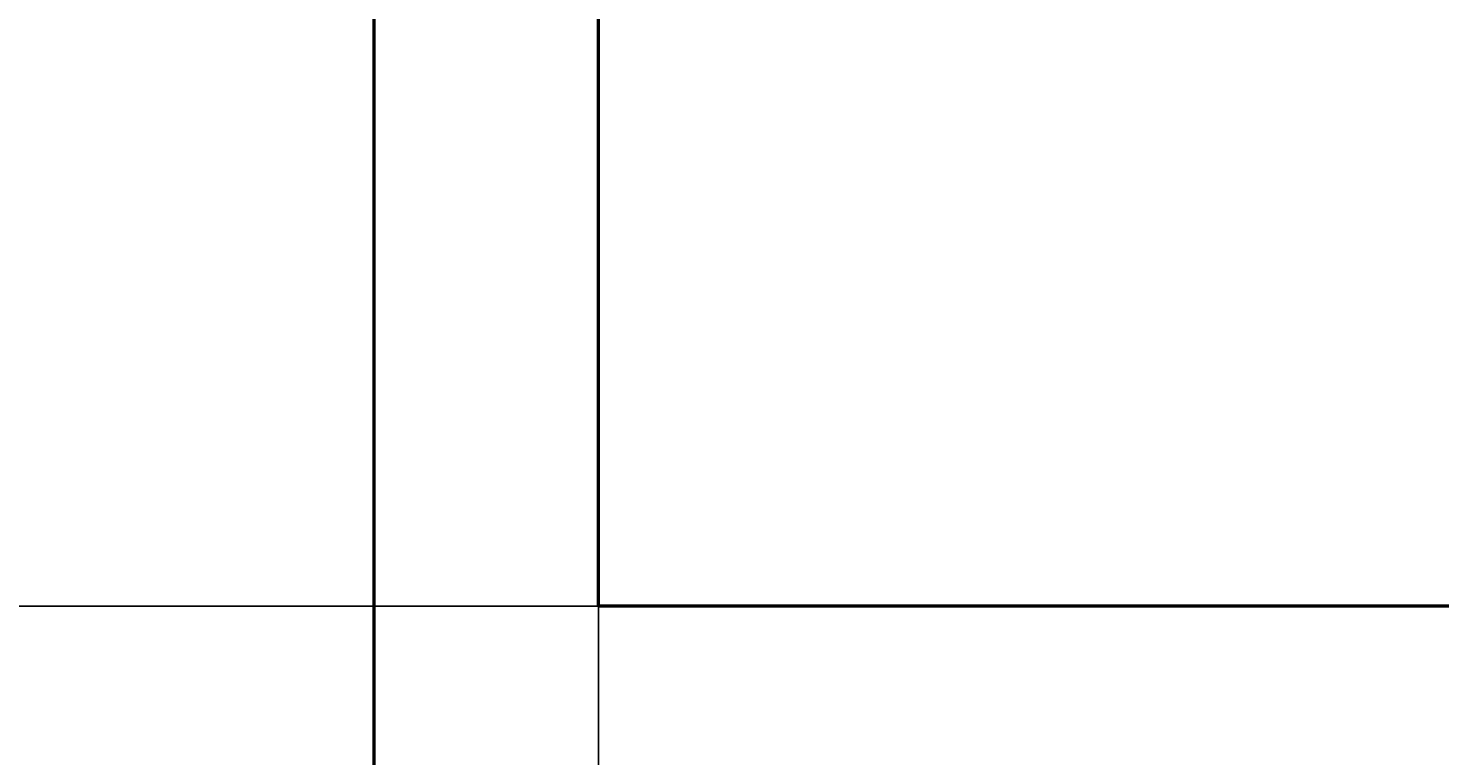
# Model space of a CAD drawing. Units: inches. Extents: x 37 to 824, y -700 to 234.
# Tile 50 of 77: x 147 to 204, y 78 to 107. Entities that reach past the tile are written whole.
import ezdxf

# ---------------------------------------------------------------- set-up
doc = ezdxf.new("R2010")
doc.units = ezdxf.units.IN
doc.header["$MEASUREMENT"] = 0
doc.layers.add('A-ANNO-DIMS', color=2, linetype='Continuous', lineweight=18)
doc.layers.add('A-WALL', color=2, linetype='Continuous', lineweight=50)
doc.styles.get("Standard").update_dxf_attribs({"font": 'arial.ttf'})
doc.dimstyles.get("Standard").update_dxf_attribs({"dimtxt": 0.18, "dimasz": 0.18, "dimexe": 0.18, "dimexo": 0.0625, "dimgap": 0.09, "dimtad": 0, "dimtih": 1, "dimtoh": 1, "dimdec": 1, "dimzin": 0, "dimdsep": 46, "dimlunit": 4, "dimtxsty": 'Standard', "dimcen": 0.09, "dimadec": 0, "dimazin": 0, "dimtfac": 1, "dimtdec": 1, "dimtofl": 0, "dimtmove": 0, "dimatfit": 3, "dimfxl": 1, "dimtolj": 1, "dimtzin": 0, "dimarcsym": 0})

# ---------------------------------------------------------------- blocks, each defined once
blk = doc.blocks.new('*D51')
at = {"layer": 'A-ANNO-DIMS', "color": 0, "lineweight": -2, "ltscale": 0.5, "transparency": 16777216}
for p, q in [((161.015, 113.09), (78.159, 113.09)), ((78.339, 112.91), (78.339, 81.772)), ((78.339, 50.27), (78.339, 81.408)), ((161.015, 50.09), (78.159, 50.09))]:
    blk.add_line(p, q, dxfattribs=at)
at = {"layer": 'A-ANNO-DIMS', "color": 0, "ltscale": 0.5, "transparency": 16777216}
for points in [[(78.309, 112.91), (78.369, 112.91), (78.339, 113.09)], [(78.309, 50.27), (78.369, 50.27), (78.339, 50.09)]]:
    blk.add_solid(points, dxfattribs=at)
at = {"layer": 'Defpoints', "color": 0, "ltscale": 0.5, "transparency": 16777216}
for p in [(161.077, 113.09), (78.339, 50.09), (161.077, 50.09)]:
    blk.add_point(p, dxfattribs=at)
at = {"layer": 'A-ANNO-DIMS', "color": 0, "ltscale": 0.5, "transparency": 16777216, "insert": (78.339, 81.59), "char_height": 0.18, "attachment_point": 5}
blk.add_mtext('\\A1;5\'-3"', dxfattribs=at)
blk = doc.blocks.new('*D60')
at = {"layer": 'A-ANNO-DIMS', "color": 0, "lineweight": -2, "ltscale": 0.5, "transparency": 16777216}
for p, q in [((419.015, 113.09), (78.159, 113.09)), ((78.339, 112.91), (78.339, 98.772)), ((78.339, 84.27), (78.339, 98.409)), ((419.015, 84.09), (78.159, 84.09))]:
    blk.add_line(p, q, dxfattribs=at)
at = {"layer": 'A-ANNO-DIMS', "color": 0, "ltscale": 0.5, "transparency": 16777216}
for points in [[(78.309, 112.91), (78.369, 112.91), (78.339, 113.09)], [(78.309, 84.27), (78.369, 84.27), (78.339, 84.09)]]:
    blk.add_solid(points, dxfattribs=at)
at = {"layer": 'Defpoints', "color": 0, "ltscale": 0.5, "transparency": 16777216}
for p in [(78.339, 113.09), (419.077, 113.09), (419.077, 84.09)]:
    blk.add_point(p, dxfattribs=at)
at = {"layer": 'A-ANNO-DIMS', "color": 0, "ltscale": 0.5, "transparency": 16777216, "insert": (78.339, 98.59), "char_height": 0.18, "attachment_point": 5}
blk.add_mtext('\\A1;2\'-5"', dxfattribs=at)
blk = doc.blocks.new('*D72')
at = {"layer": 'A-ANNO-DIMS', "color": 0, "lineweight": -2, "ltscale": 0.5, "transparency": 16777216}
for p, q in [((170.077, 84.153), (170.077, 234.17)), ((170.257, 233.99), (209.804, 233.99)), ((250.01, 233.99), (210.463, 233.99)), ((250.19, 84.153), (250.19, 234.17))]:
    blk.add_line(p, q, dxfattribs=at)
at = {"layer": 'A-ANNO-DIMS', "color": 0, "ltscale": 0.5, "transparency": 16777216}
for points in [[(170.257, 234.02), (170.257, 233.96), (170.077, 233.99)], [(250.01, 234.02), (250.01, 233.96), (250.19, 233.99)]]:
    blk.add_solid(points, dxfattribs=at)
at = {"layer": 'Defpoints', "color": 0, "ltscale": 0.5, "transparency": 16777216}
for p in [(250.19, 233.99), (170.077, 84.09), (250.19, 84.09)]:
    blk.add_point(p, dxfattribs=at)
at = {"layer": 'A-ANNO-DIMS', "color": 0, "ltscale": 0.5, "transparency": 16777216, "insert": (210.133, 233.99), "char_height": 0.18, "attachment_point": 5}
blk.add_mtext('\\A1;6\'-8"', dxfattribs=at)
blk = doc.blocks.new('*D84')
at = {"layer": 'A-ANNO-DIMS', "color": 0, "lineweight": -2, "ltscale": 0.5, "transparency": 16777216}
for p, q in [((170.077, -265.847), (170.077, 234.17)), ((170.257, 233.99), (189.748, 233.99)), ((209.897, 233.99), (190.406, 233.99)), ((210.077, -265.847), (210.077, 234.17))]:
    blk.add_line(p, q, dxfattribs=at)
at = {"layer": 'A-ANNO-DIMS', "color": 0, "ltscale": 0.5, "transparency": 16777216}
for points in [[(170.257, 234.02), (170.257, 233.96), (170.077, 233.99)], [(209.897, 234.02), (209.897, 233.96), (210.077, 233.99)]]:
    blk.add_solid(points, dxfattribs=at)
at = {"layer": 'Defpoints', "color": 0, "ltscale": 0.5, "transparency": 16777216}
for p in [(210.077, 233.99), (170.077, -265.91), (210.077, -265.91)]:
    blk.add_point(p, dxfattribs=at)
at = {"layer": 'A-ANNO-DIMS', "color": 0, "ltscale": 0.5, "transparency": 16777216, "insert": (190.077, 233.99), "char_height": 0.18, "attachment_point": 5}
blk.add_mtext('\\A1;3\'-4"', dxfattribs=at)
blk = doc.blocks.new('*D85')
at = {"layer": 'A-ANNO-DIMS', "color": 0, "lineweight": -2, "ltscale": 0.5, "transparency": 16777216}
for p, q in [((170.077, -356.847), (170.077, 234.17)), ((170.257, 233.99), (187.748, 233.99)), ((205.897, 233.99), (188.406, 233.99)), ((206.077, -356.847), (206.077, 234.17))]:
    blk.add_line(p, q, dxfattribs=at)
at = {"layer": 'A-ANNO-DIMS', "color": 0, "ltscale": 0.5, "transparency": 16777216}
for points in [[(170.257, 234.02), (170.257, 233.96), (170.077, 233.99)], [(205.897, 234.02), (205.897, 233.96), (206.077, 233.99)]]:
    blk.add_solid(points, dxfattribs=at)
at = {"layer": 'Defpoints', "color": 0, "ltscale": 0.5, "transparency": 16777216}
for p in [(206.077, 233.99), (170.077, -356.91), (206.077, -356.91)]:
    blk.add_point(p, dxfattribs=at)
at = {"layer": 'A-ANNO-DIMS', "color": 0, "ltscale": 0.5, "transparency": 16777216, "insert": (188.077, 233.99), "char_height": 0.18, "attachment_point": 5}
blk.add_mtext('\\A1;3\'-0"', dxfattribs=at)

msp = doc.modelspace()

# ---------------------------------------------------------------- linework, layer by layer
at = {"layer": 'A-WALL'}
for p, q in [((161.077, 75.09), (161.077, 191.09)), ((170.077, 84.09), (170.077, 182.09)), ((250.19, 84.09), (170.077, 84.09))]:
    msp.add_line(p, q, dxfattribs=at)

# ---------------------------------------------------------------- dimensions: what is measured, and where the dimension line sits
at = {"layer": 'A-ANNO-DIMS', "ltscale": 0.5}
for base, p1, p2, picture, middle in [((250.19, 233.99), (170.077, 84.09), (250.19, 84.09), '*D72', (210.133, 233.99)), ((210.077, 233.99), (170.077, -265.91), (210.077, -265.91), '*D84', (190.077, 233.99)), ((206.077, 233.99), (170.077, -356.91), (206.077, -356.91), '*D85', (188.077, 233.99))]:
    dim = msp.add_linear_dim(base=base, p1=p1, p2=p2, dimstyle='Standard', override={"dimdec": 1, "dimlfac": 1, "dimrnd": 0, "dimzin": 1, "dimdsep": 46, "dimlunit": 4, "dimfrac": 2}, dxfattribs=at)
    dim.commit()
    dim.dimension.update_dxf_attribs({"geometry": picture, "text_midpoint": middle})
for base, p1, p2, picture, middle in [((78.339, 50.09), (161.077, 113.09), (161.077, 50.09), '*D51', (78.339, 81.59)), ((78.339, 113.09), (419.077, 84.09), (419.077, 113.09), '*D60', (78.339, 98.59))]:
    dim = msp.add_linear_dim(base=base, p1=p1, p2=p2, angle=90, dimstyle='Standard', override={"dimdec": 1, "dimlfac": 1, "dimrnd": 0, "dimzin": 1, "dimdsep": 46, "dimlunit": 4, "dimfrac": 2}, dxfattribs=at)
    dim.commit()
    dim.dimension.update_dxf_attribs({"geometry": picture, "text_midpoint": middle})

doc.saveas('drawing.dxf')
